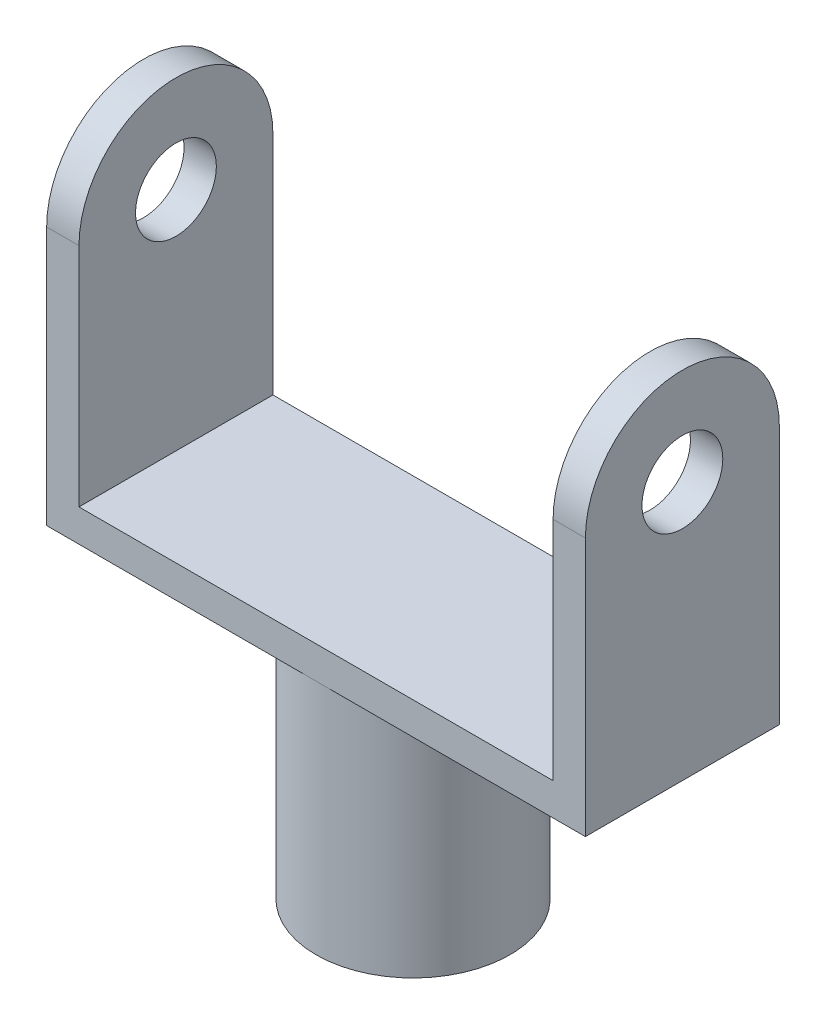
from build123d import *

# Parameters (mm, degrees)
STEM_PROFILE_36_R           = 18
STEM_36X44_DEPTH            = 44
BASE_PLATE_PROFILE_W        = 88
BASE_PLATE_PROFILE_H        = 36
BASE_PLATE_88X36X6_DEPTH    = 6
LUG_PROFILE_WITH_PIN_HOLE_R = 7.5
LUG_6MM_DEPTH               = 6


with BuildPart() as part:
    # Stem Profile Ø36 → Stem Ø36x44 (new body)
    with BuildSketch(Plane(origin=(0, 0, 0), x_dir=(1, 0, 0), z_dir=(0, 1, 0))):
        with Locations(Location((0, 0, 0), (0, 0, 270))):
            Circle(STEM_PROFILE_36_R)
    extrude(amount=STEM_36X44_DEPTH)

    # Base Plate Profile → Base Plate 88x36x6 (add)
    with BuildSketch(Plane(origin=(0, 44, 0), x_dir=(1, 0, 0), z_dir=(0, 1, 0))):
        Rectangle(BASE_PLATE_PROFILE_W, BASE_PLATE_PROFILE_H)
    extrude(amount=BASE_PLATE_88X36X6_DEPTH)

    # Lug Profile with Pin Hole → Lug 6mm (add)
    with BuildSketch(Plane(origin=(44, 0, 0), x_dir=(0, 0, -1), z_dir=(1, 0, 0))):
        with BuildLine():
            Line((-18, 44), (18, 44))
            Line((18, 44), (18, 92))
            ThreePointArc((18, 92), (0, 110), (-18, 92))
            Line((-18, 92), (-18, 44))
        make_face()
        with Locations((0, 92)):
            Circle(LUG_PROFILE_WITH_PIN_HOLE_R, mode=Mode.SUBTRACT)
    lug_6mm = extrude(amount=LUG_6MM_DEPTH)

    # Lug Mirror: Lug 6mm across plane
    add(lug_6mm.mirror(Plane(origin=(0, 0, 0), x_dir=(0, 0, 1), z_dir=(1, 0, 0))))


solid = part.part
